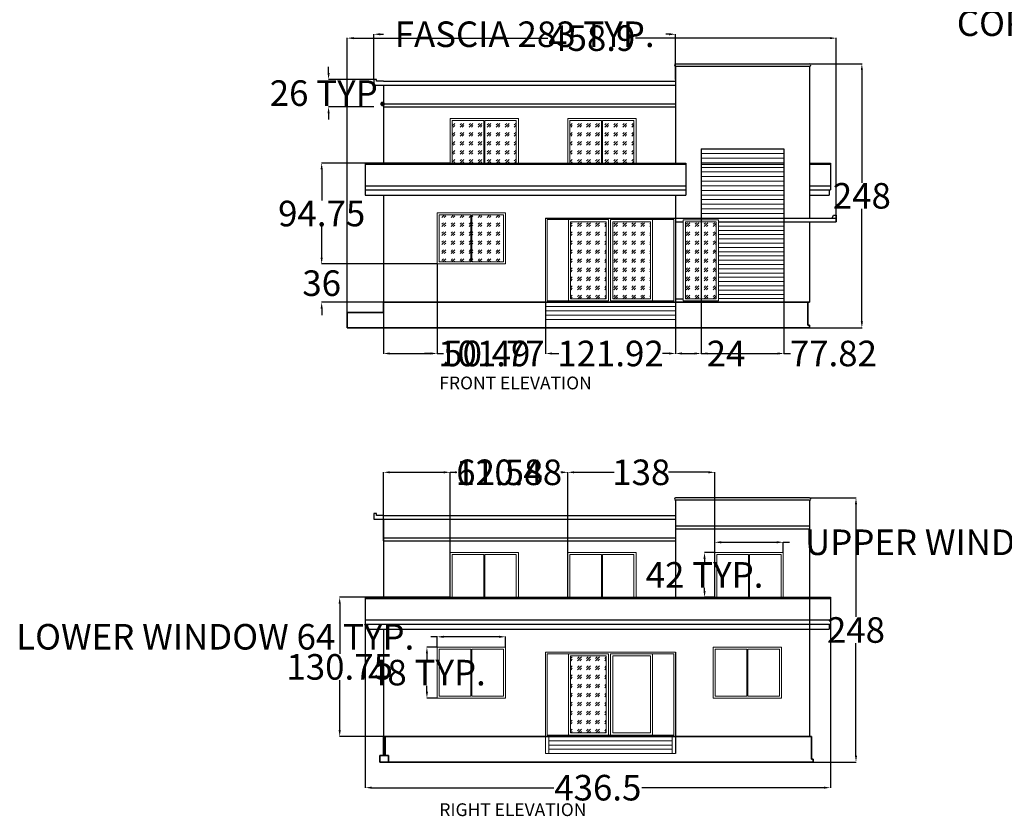
# Model space of a CAD drawing. Units: inches. Extents: x -15 to 1815, y 1023 to 2303.
# Tile 1 of 8: x -15 to 910, y 1024 to 1772. Entities that reach past the tile are written whole.
import ezdxf

# ---------------------------------------------------------------- set-up
doc = ezdxf.new("R2010")
doc.units = ezdxf.units.IN
doc.header["$MEASUREMENT"] = 0
for name, color, linetype, lineweight in [('A-ANNO-DIMS', 2, 'Continuous', 18), ('A-ANNO-TEXT', 7, 'Continuous', 25), ('A-DOOR', 3, 'Continuous', 18), ('A-ELEV', 7, 'Continuous', 25), ('A-ELEV-PATT', 252, 'Continuous', 13), ('A-FLOR-STRS', 3, 'Continuous', 18), ('A-GLAZ', 4, 'Continuous', 18), ('A-GLAZ-PATT', 252, 'Continuous', 13), ('A-ROOF', 7, 'Continuous', 25), ('S-FNDN', 7, 'Continuous', 35)]:
    doc.layers.add(name, color=color, linetype=linetype, lineweight=lineweight)
doc.styles.get("Standard").update_dxf_attribs({"font": 'arial.ttf'})
doc.dimstyles.get("Standard").update_dxf_attribs({"dimtxt": 24, "dimasz": 6, "dimexe": 0.18, "dimexo": 0.0625, "dimgap": 0.09, "dimtad": 0, "dimtih": 1, "dimtoh": 1, "dimdec": 0, "dimzin": 0, "dimdsep": 46, "dimlunit": 3, "dimtxsty": 'Standard', "dimcen": 0.09, "dimadec": 0, "dimazin": 0, "dimtfac": 1, "dimtdec": 0, "dimtofl": 0, "dimtmove": 0, "dimatfit": 3, "dimfxl": 1, "dimtolj": 1, "dimtzin": 0, "dimarcsym": 0})
pattern_1 = [(45, (0, 0), (8.485281, 0), [5, -7]), (45, (2.1213, 0), (8.485281, 0), [2, -10]), (45, (0, 2.1213), (8.485281, 0), [2, -10])]

# ---------------------------------------------------------------- blocks, each defined once
blk = doc.blocks.new('WIN-TWIN-ELEV-42')
for p, q in [((0, 42), (64.17, 42)), ((0, 42), (0, 0)), ((2, 40), (31.58, 40)), ((2, 40), (2, 0)), ((31.58, 0), (31.58, 40)), ((32.58, 40), (62.17, 40)), ((32.58, 0), (32.58, 40)), ((62.17, 40), (62.17, 0)), ((64.17, 42), (64.17, 0))]:
    blk.add_line(p, q)
blk = doc.blocks.new('WIN-TWIN-ELEV-48')
for p, q in [((0, 48), (64.17, 48)), ((0, 48), (0, 0)), ((64.17, 48), (64.17, 0)), ((2, 46), (31.58, 46)), ((2, 46), (2, 2)), ((31.58, 2), (31.58, 46)), ((32.58, 2), (32.58, 46)), ((32.58, 46), (62.17, 46)), ((62.17, 46), (62.17, 2)), ((0, 0), (64.17, 0)), ((2, 2), (31.58, 2)), ((32.58, 2), (62.17, 2))]:
    blk.add_line(p, q)
blk = doc.blocks.new('COPING-ROUND-END')
for p, q in [((1.07, 2.13), (126.89, 2.13)), ((1.07, 0), (126.89, 0))]:
    blk.add_line(p, q)
for centre, start, end in [((1.07, 1.07), 90, 270), ((126.89, 1.07), 270, 90)]:
    blk.add_arc(centre, 1.07, start, end)
blk = doc.blocks.new('FASCIA-PARAPET-ELEV')
for p, q in [((2.47, 25.64), (0, 25.64)), ((0, 25.64), (0, 20.39)), ((0, 20.39), (283.12, 20.39)), ((2.47, 23.92), (2.47, 25.64)), ((8.95, 23.92), (2.47, 23.92)), ((8.95, 23.92), (283.12, 23.92)), ((8.95, 2.89), (283.12, 2.89)), ((8.95, 0), (283.12, 0))]:
    blk.add_line(p, q)
blk = doc.blocks.new('*D41')
at = {"layer": 'A-ANNO-DIMS', "color": 0, "lineweight": -2, "transparency": 16777216}
for p, q in [((637.91, 1272.2), (637.91, 1281.94)), ((643.91, 1281.76), (696.08, 1281.76)), ((702.08, 1272.2), (702.08, 1281.94)), ((702.08, 1281.76), (708.08, 1281.76))]:
    blk.add_line(p, q, dxfattribs=at)
at = {"layer": 'A-ANNO-DIMS', "color": 0, "transparency": 16777216}
for points in [[(643.91, 1282.76), (643.91, 1280.76), (637.91, 1281.76)], [(696.08, 1282.76), (696.08, 1280.76), (702.08, 1281.76)]]:
    blk.add_solid(points, dxfattribs=at)
at = {"layer": 'Defpoints', "color": 0, "transparency": 16777216}
for p in [(702.08, 1281.76), (637.91, 1272.13), (702.08, 1272.13)]:
    blk.add_point(p, dxfattribs=at)
at = {"layer": 'A-ANNO-DIMS', "color": 0, "transparency": 16777216, "insert": (906.58, 1281.76), "char_height": 24, "attachment_point": 5}
blk.add_mtext('\\A1;UPPER WINDOW 64 TYP.', dxfattribs=at)
blk = doc.blocks.new('*D42')
at = {"layer": 'A-ANNO-DIMS', "color": 0, "lineweight": -2, "transparency": 16777216}
for p, q in [((637.85, 1272.13), (628.11, 1272.13)), ((628.29, 1266.13), (628.29, 1263.28)), ((628.29, 1236.13), (628.29, 1238.99)), ((637.85, 1230.13), (628.11, 1230.13))]:
    blk.add_line(p, q, dxfattribs=at)
at = {"layer": 'A-ANNO-DIMS', "color": 0, "transparency": 16777216}
for points in [[(627.29, 1266.13), (629.29, 1266.13), (628.29, 1272.13)], [(627.29, 1236.13), (629.29, 1236.13), (628.29, 1230.13)]]:
    blk.add_solid(points, dxfattribs=at)
at = {"layer": 'Defpoints', "color": 0, "transparency": 16777216}
for p in [(628.29, 1272.13), (637.91, 1272.13), (637.91, 1230.13)]:
    blk.add_point(p, dxfattribs=at)
at = {"layer": 'A-ANNO-DIMS', "color": 0, "transparency": 16777216, "insert": (628.29, 1251.13), "char_height": 24, "attachment_point": 5}
blk.add_mtext('\\A1;42 TYP.', dxfattribs=at)
blk = doc.blocks.new('*D43')
at = {"layer": 'A-ANNO-DIMS', "color": 0, "lineweight": -2, "transparency": 16777216}
for p, q in [((377.32, 1193.01), (371.32, 1193.01)), ((377.32, 1183.44), (377.32, 1193.19)), ((435.49, 1193.01), (383.32, 1193.01)), ((441.49, 1183.44), (441.49, 1193.19))]:
    blk.add_line(p, q, dxfattribs=at)
at = {"layer": 'A-ANNO-DIMS', "color": 0, "transparency": 16777216}
for points in [[(383.32, 1194.01), (383.32, 1192.01), (377.32, 1193.01)], [(435.49, 1194.01), (435.49, 1192.01), (441.49, 1193.01)]]:
    blk.add_solid(points, dxfattribs=at)
at = {"layer": 'Defpoints', "color": 0, "transparency": 16777216}
for p in [(377.32, 1193.01), (377.32, 1183.38), (441.49, 1183.38)]:
    blk.add_point(p, dxfattribs=at)
at = {"layer": 'A-ANNO-DIMS', "color": 0, "transparency": 16777216, "insert": (169.01, 1193.01), "char_height": 24, "attachment_point": 5}
blk.add_mtext('\\A1;LOWER WINDOW 64 TYP.', dxfattribs=at)
blk = doc.blocks.new('*D44')
at = {"layer": 'A-ANNO-DIMS', "color": 0, "lineweight": -2, "transparency": 16777216}
for p, q in [((377.26, 1183.38), (367.52, 1183.38)), ((367.7, 1177.38), (367.7, 1171.73)), ((367.7, 1141.38), (367.7, 1147.04)), ((377.26, 1135.38), (367.52, 1135.38))]:
    blk.add_line(p, q, dxfattribs=at)
at = {"layer": 'A-ANNO-DIMS', "color": 0, "transparency": 16777216}
for points in [[(366.7, 1177.38), (368.7, 1177.38), (367.7, 1183.38)], [(366.7, 1141.38), (368.7, 1141.38), (367.7, 1135.38)]]:
    blk.add_solid(points, dxfattribs=at)
at = {"layer": 'Defpoints', "color": 0, "transparency": 16777216}
for p in [(377.32, 1183.38), (367.7, 1135.38), (377.32, 1135.38)]:
    blk.add_point(p, dxfattribs=at)
at = {"layer": 'A-ANNO-DIMS', "color": 0, "transparency": 16777216, "insert": (367.7, 1159.38), "char_height": 24, "attachment_point": 5}
blk.add_mtext('\\A1;48 TYP.', dxfattribs=at)
blk = doc.blocks.new('*D45')
at = {"layer": 'A-ANNO-DIMS', "color": 0, "lineweight": -2, "transparency": 16777216}
for p, q in [((1138.43, 1769.16), (1132.43, 1769.16)), ((1138.43, 1750.02), (1138.43, 1769.34)), ((1260.44, 1769.16), (1144.43, 1769.16)), ((1266.44, 1750.02), (1266.44, 1769.34))]:
    blk.add_line(p, q, dxfattribs=at)
at = {"layer": 'A-ANNO-DIMS', "color": 0, "transparency": 16777216}
for points in [[(1144.43, 1770.16), (1144.43, 1768.16), (1138.43, 1769.16)], [(1260.44, 1770.16), (1260.44, 1768.16), (1266.44, 1769.16)]]:
    blk.add_solid(points, dxfattribs=at)
at = {"layer": 'Defpoints', "color": 0, "transparency": 16777216}
for p in [(1138.43, 1769.16), (1138.43, 1749.96), (1266.44, 1749.96)]:
    blk.add_point(p, dxfattribs=at)
at = {"layer": 'A-ANNO-DIMS', "color": 0, "transparency": 16777216, "insert": (993.96, 1769.16), "char_height": 24, "attachment_point": 5}
blk.add_mtext('\\A1;COPING 128 TYP.', dxfattribs=at)
blk = doc.blocks.new('*D57')
at = {"layer": 'A-ANNO-DIMS', "color": 0, "lineweight": -2, "transparency": 16777216}
for p, q in [((317.89, 1716.39), (317.89, 1758.98)), ((323.89, 1758.8), (327.1, 1758.8)), ((595.01, 1758.8), (591.8, 1758.8)), ((601.01, 1716.39), (601.01, 1758.98))]:
    blk.add_line(p, q, dxfattribs=at)
at = {"layer": 'A-ANNO-DIMS', "color": 0, "transparency": 16777216}
for points in [[(323.89, 1759.8), (323.89, 1757.8), (317.89, 1758.8)], [(595.01, 1759.8), (595.01, 1757.8), (601.01, 1758.8)]]:
    blk.add_solid(points, dxfattribs=at)
at = {"layer": 'Defpoints', "color": 0, "transparency": 16777216}
for p in [(601.01, 1758.8), (317.89, 1716.33), (601.01, 1716.33)]:
    blk.add_point(p, dxfattribs=at)
at = {"layer": 'A-ANNO-DIMS', "color": 0, "transparency": 16777216, "insert": (459.45, 1758.8), "char_height": 24, "attachment_point": 5}
blk.add_mtext('\\A1;FASCIA 283 TYP.', dxfattribs=at)
blk = doc.blocks.new('*D58')
at = {"layer": 'A-ANNO-DIMS', "color": 0, "lineweight": -2, "transparency": 16777216}
for p, q in [((275.42, 1722.33), (275.42, 1728.33)), ((317.83, 1716.33), (275.24, 1716.33)), ((317.83, 1690.69), (275.24, 1690.69)), ((275.42, 1684.69), (275.42, 1678.69))]:
    blk.add_line(p, q, dxfattribs=at)
at = {"layer": 'A-ANNO-DIMS', "color": 0, "transparency": 16777216}
for points in [[(274.42, 1722.33), (276.42, 1722.33), (275.42, 1716.33)], [(274.42, 1684.69), (276.42, 1684.69), (275.42, 1690.69)]]:
    blk.add_solid(points, dxfattribs=at)
at = {"layer": 'Defpoints', "color": 0, "transparency": 16777216}
for p in [(275.42, 1716.33), (317.89, 1716.33), (317.89, 1690.69)]:
    blk.add_point(p, dxfattribs=at)
at = {"layer": 'A-ANNO-DIMS', "color": 0, "transparency": 16777216, "insert": (275.42, 1703.51), "char_height": 24, "attachment_point": 5}
blk.add_mtext('\\A1;26 TYP.', dxfattribs=at)
blk = doc.blocks.new('*D88')
at = {"layer": 'A-ANNO-DIMS', "color": 0, "lineweight": -2, "transparency": 16777216}
for p, q in [((292.98, 1483.14), (292.98, 1755.33)), ((298.98, 1755.15), (481.34, 1755.15)), ((745.89, 1755.15), (563.53, 1755.15)), ((751.89, 1589.12), (751.89, 1755.33))]:
    blk.add_line(p, q, dxfattribs=at)
at = {"layer": 'A-ANNO-DIMS', "color": 0, "transparency": 16777216}
for points in [[(298.98, 1756.15), (298.98, 1754.15), (292.98, 1755.15)], [(745.89, 1756.15), (745.89, 1754.15), (751.89, 1755.15)]]:
    blk.add_solid(points, dxfattribs=at)
at = {"layer": 'Defpoints', "color": 0, "transparency": 16777216}
for p in [(751.89, 1755.15), (751.89, 1589.05), (292.98, 1483.08)]:
    blk.add_point(p, dxfattribs=at)
at = {"layer": 'A-ANNO-DIMS', "color": 0, "transparency": 16777216, "insert": (522.44, 1755.15), "char_height": 24, "attachment_point": 5}
blk.add_mtext('\\A1;458.9', dxfattribs=at)
blk = doc.blocks.new('*D89')
at = {"layer": 'A-ANNO-DIMS', "color": 0, "lineweight": -2, "transparency": 16777216}
for p, q in [((726.9, 1731.1), (776.12, 1731.1)), ((775.94, 1725.1), (775.94, 1619.43)), ((775.94, 1489.08), (775.94, 1594.75)), ((726.9, 1483.08), (776.12, 1483.08))]:
    blk.add_line(p, q, dxfattribs=at)
at = {"layer": 'A-ANNO-DIMS', "color": 0, "transparency": 16777216}
for points in [[(774.94, 1725.1), (776.94, 1725.1), (775.94, 1731.1)], [(774.94, 1489.08), (776.94, 1489.08), (775.94, 1483.08)]]:
    blk.add_solid(points, dxfattribs=at)
at = {"layer": 'Defpoints', "color": 0, "transparency": 16777216}
for p in [(726.83, 1731.1), (775.94, 1731.1), (726.83, 1483.08)]:
    blk.add_point(p, dxfattribs=at)
at = {"layer": 'A-ANNO-DIMS', "color": 0, "transparency": 16777216, "insert": (775.94, 1607.09), "char_height": 24, "attachment_point": 5}
blk.add_mtext('\\A1;248', dxfattribs=at)
blk = doc.blocks.new('*D90')
at = {"layer": 'A-ANNO-DIMS', "color": 0, "lineweight": -2, "transparency": 16777216}
for p, q in [((377.32, 1543.01), (377.32, 1458.85)), ((326.83, 1507.01), (326.83, 1458.85)), ((332.83, 1459.03), (371.32, 1459.03)), ((377.32, 1459.03), (383.32, 1459.03))]:
    blk.add_line(p, q, dxfattribs=at)
at = {"layer": 'A-ANNO-DIMS', "color": 0, "transparency": 16777216}
for points in [[(332.83, 1460.03), (332.83, 1458.03), (326.83, 1459.03)], [(371.32, 1460.03), (371.32, 1458.03), (377.32, 1459.03)]]:
    blk.add_solid(points, dxfattribs=at)
at = {"layer": 'Defpoints', "color": 0, "transparency": 16777216}
for p in [(377.32, 1543.08), (326.83, 1507.08), (377.32, 1459.03)]:
    blk.add_point(p, dxfattribs=at)
at = {"layer": 'A-ANNO-DIMS', "color": 0, "transparency": 16777216, "insert": (423.93, 1459.03), "char_height": 24, "attachment_point": 5}
blk.add_mtext('\\A1;50.49', dxfattribs=at)
blk = doc.blocks.new('*D91')
at = {"layer": 'A-ANNO-DIMS', "color": 0, "lineweight": -2, "transparency": 16777216}
for p, q in [((377.320354, 1543.014849), (377.320354, 1458.847349)), ((479.094066, 1507.014849), (479.094066, 1458.847349)), ((371.320354, 1459.027349), (365.320354, 1459.027349)), ((485.094066, 1459.027349), (491.094066, 1459.027349))]:
    blk.add_line(p, q, dxfattribs=at)
at = {"layer": 'A-ANNO-DIMS', "color": 0, "transparency": 16777216}
for points in [[(371.320354, 1460.027349), (371.320354, 1458.027349), (377.320354, 1459.027349)], [(485.094066, 1460.027349), (485.094066, 1458.027349), (479.094066, 1459.027349)]]:
    blk.add_solid(points, dxfattribs=at)
at = {"layer": 'Defpoints', "color": 0, "transparency": 16777216}
for p in [(377.320354, 1543.077349), (479.094066, 1507.077349), (479.094066, 1459.027349)]:
    blk.add_point(p, dxfattribs=at)
at = {"layer": 'A-ANNO-DIMS', "color": 0, "transparency": 16777216, "insert": (428.20721, 1459.027349), "char_height": 24, "attachment_point": 5}
blk.add_mtext('\\A1;101.77', dxfattribs=at)
blk = doc.blocks.new('*D92')
at = {"layer": 'A-ANNO-DIMS', "color": 0, "lineweight": -2, "transparency": 16777216}
for p, q in [((479.09, 1507.01), (479.09, 1458.85)), ((601.01, 1507.01), (601.01, 1458.85)), ((485.09, 1459.03), (491.4, 1459.03)), ((595.01, 1459.03), (588.71, 1459.03))]:
    blk.add_line(p, q, dxfattribs=at)
at = {"layer": 'A-ANNO-DIMS', "color": 0, "transparency": 16777216}
for points in [[(485.09, 1460.03), (485.09, 1458.03), (479.09, 1459.03)], [(595.01, 1460.03), (595.01, 1458.03), (601.01, 1459.03)]]:
    blk.add_solid(points, dxfattribs=at)
at = {"layer": 'Defpoints', "color": 0, "transparency": 16777216}
for p in [(479.09, 1507.08), (601.01, 1507.08), (601.01, 1459.03)]:
    blk.add_point(p, dxfattribs=at)
at = {"layer": 'A-ANNO-DIMS', "color": 0, "transparency": 16777216, "insert": (540.05, 1459.03), "char_height": 24, "attachment_point": 5}
blk.add_mtext('\\A1;121.92', dxfattribs=at)
blk = doc.blocks.new('*D93')
at = {"layer": 'A-ANNO-DIMS', "color": 0, "lineweight": -2, "transparency": 16777216}
for p, q in [((625.01, 1651.01), (625.01, 1458.85)), ((601.01, 1507.01), (601.01, 1458.85)), ((607.01, 1459.03), (619.01, 1459.03)), ((625.01, 1459.03), (631.01, 1459.03))]:
    blk.add_line(p, q, dxfattribs=at)
at = {"layer": 'A-ANNO-DIMS', "color": 0, "transparency": 16777216}
for points in [[(607.01, 1460.03), (607.01, 1458.03), (601.01, 1459.03)], [(619.01, 1460.03), (619.01, 1458.03), (625.01, 1459.03)]]:
    blk.add_solid(points, dxfattribs=at)
at = {"layer": 'Defpoints', "color": 0, "transparency": 16777216}
for p in [(625.01, 1651.08), (601.01, 1507.08), (625.01, 1459.03)]:
    blk.add_point(p, dxfattribs=at)
at = {"layer": 'A-ANNO-DIMS', "color": 0, "transparency": 16777216, "insert": (648.45, 1459.03), "char_height": 24, "attachment_point": 5}
blk.add_mtext('\\A1;24', dxfattribs=at)
blk = doc.blocks.new('*D94')
at = {"layer": 'A-ANNO-DIMS', "color": 0, "lineweight": -2, "transparency": 16777216}
for p, q in [((625.01, 1651.01), (625.01, 1458.85)), ((702.83, 1507.01), (702.83, 1458.85)), ((631.01, 1459.03), (696.83, 1459.03)), ((702.83, 1459.03), (708.83, 1459.03))]:
    blk.add_line(p, q, dxfattribs=at)
at = {"layer": 'A-ANNO-DIMS', "color": 0, "transparency": 16777216}
for points in [[(631.01, 1460.03), (631.01, 1458.03), (625.01, 1459.03)], [(696.83, 1460.03), (696.83, 1458.03), (702.83, 1459.03)]]:
    blk.add_solid(points, dxfattribs=at)
at = {"layer": 'Defpoints', "color": 0, "transparency": 16777216}
for p in [(625.01, 1651.08), (702.83, 1507.08), (702.83, 1459.03)]:
    blk.add_point(p, dxfattribs=at)
at = {"layer": 'A-ANNO-DIMS', "color": 0, "transparency": 16777216, "insert": (749.2, 1459.03), "char_height": 24, "attachment_point": 5}
blk.add_mtext('\\A1;77.82', dxfattribs=at)
blk = doc.blocks.new('*D95')
at = {"layer": 'A-ANNO-DIMS', "color": 0, "lineweight": -2, "transparency": 16777216}
for p, q in [((268.932113, 1549.077349), (268.932113, 1555.077349)), ((377.257854, 1543.077349), (268.752113, 1543.077349)), ((326.772175, 1507.077349), (268.752113, 1507.077349)), ((268.932113, 1501.077349), (268.932113, 1495.077349))]:
    blk.add_line(p, q, dxfattribs=at)
at = {"layer": 'A-ANNO-DIMS', "color": 0, "transparency": 16777216}
for points in [[(267.932113, 1549.077349), (269.932113, 1549.077349), (268.932113, 1543.077349)], [(267.932113, 1501.077349), (269.932113, 1501.077349), (268.932113, 1507.077349)]]:
    blk.add_solid(points, dxfattribs=at)
at = {"layer": 'Defpoints', "color": 0, "transparency": 16777216}
for p in [(268.932113, 1543.077349), (377.320354, 1543.077349), (326.834675, 1507.077349)]:
    blk.add_point(p, dxfattribs=at)
at = {"layer": 'A-ANNO-DIMS', "color": 0, "transparency": 16777216, "insert": (268.932113, 1525.077349), "char_height": 24, "attachment_point": 5}
blk.add_mtext('\\A1;36', dxfattribs=at)
blk = doc.blocks.new('*D96')
at = {"layer": 'A-ANNO-DIMS', "color": 0, "lineweight": -2, "transparency": 16777216}
for p, q in [((389.35, 1637.83), (268.75, 1637.83)), ((268.93, 1631.83), (268.93, 1602.8)), ((268.93, 1549.08), (268.93, 1578.11)), ((377.26, 1543.08), (268.75, 1543.08))]:
    blk.add_line(p, q, dxfattribs=at)
at = {"layer": 'A-ANNO-DIMS', "color": 0, "transparency": 16777216}
for points in [[(267.93, 1631.83), (269.93, 1631.83), (268.93, 1637.83)], [(267.93, 1549.08), (269.93, 1549.08), (268.93, 1543.08)]]:
    blk.add_solid(points, dxfattribs=at)
at = {"layer": 'Defpoints', "color": 0, "transparency": 16777216}
for p in [(268.93, 1637.83), (389.41, 1637.83), (377.32, 1543.08)]:
    blk.add_point(p, dxfattribs=at)
at = {"layer": 'A-ANNO-DIMS', "color": 0, "transparency": 16777216, "insert": (268.93, 1590.45), "char_height": 24, "attachment_point": 5}
blk.add_mtext('\\A1;94.75', dxfattribs=at)
blk = doc.blocks.new('*D97')
at = {"layer": 'A-ANNO-DIMS', "color": 0, "lineweight": -2, "transparency": 16777216}
for p, q in [((309.87, 1230.07), (309.87, 1051.15)), ((746.38, 1230.07), (746.38, 1051.15)), ((315.87, 1051.33), (486.97, 1051.33)), ((740.38, 1051.33), (569.28, 1051.33))]:
    blk.add_line(p, q, dxfattribs=at)
at = {"layer": 'A-ANNO-DIMS', "color": 0, "transparency": 16777216}
for points in [[(315.87, 1052.33), (315.87, 1050.33), (309.87, 1051.33)], [(740.38, 1052.33), (740.38, 1050.33), (746.38, 1051.33)]]:
    blk.add_solid(points, dxfattribs=at)
at = {"layer": 'Defpoints', "color": 0, "transparency": 16777216}
for p in [(309.87, 1230.13), (746.38, 1230.13), (746.38, 1051.33)]:
    blk.add_point(p, dxfattribs=at)
at = {"layer": 'A-ANNO-DIMS', "color": 0, "transparency": 16777216, "insert": (528.13, 1051.33), "char_height": 24, "attachment_point": 5}
blk.add_mtext('\\A1;436.5', dxfattribs=at)
blk = doc.blocks.new('*D98')
at = {"layer": 'A-ANNO-DIMS', "color": 0, "lineweight": -2, "transparency": 16777216}
for p, q in [((726.9, 1323.41), (770.61, 1323.41)), ((770.43, 1317.41), (770.43, 1211.74)), ((770.43, 1081.38), (770.43, 1187.05)), ((730.36, 1075.38), (770.61, 1075.38))]:
    blk.add_line(p, q, dxfattribs=at)
at = {"layer": 'A-ANNO-DIMS', "color": 0, "transparency": 16777216}
for points in [[(769.43, 1317.41), (771.43, 1317.41), (770.43, 1323.41)], [(769.43, 1081.38), (771.43, 1081.38), (770.43, 1075.38)]]:
    blk.add_solid(points, dxfattribs=at)
at = {"layer": 'Defpoints', "color": 0, "transparency": 16777216}
for p in [(726.83, 1323.41), (770.43, 1323.41), (730.3, 1075.38)]:
    blk.add_point(p, dxfattribs=at)
at = {"layer": 'A-ANNO-DIMS', "color": 0, "transparency": 16777216, "insert": (770.43, 1199.39), "char_height": 24, "attachment_point": 5}
blk.add_mtext('\\A1;248', dxfattribs=at)
blk = doc.blocks.new('*D99')
at = {"layer": 'A-ANNO-DIMS', "color": 0, "lineweight": -2, "transparency": 16777216}
for p, q in [((326.83, 1283.06), (326.83, 1347.64)), ((332.83, 1347.46), (383.41, 1347.46)), ((389.41, 1230.2), (389.41, 1347.64)), ((389.41, 1347.46), (395.41, 1347.46))]:
    blk.add_line(p, q, dxfattribs=at)
at = {"layer": 'A-ANNO-DIMS', "color": 0, "transparency": 16777216}
for points in [[(332.83, 1348.46), (332.83, 1346.46), (326.83, 1347.46)], [(383.41, 1348.46), (383.41, 1346.46), (389.41, 1347.46)]]:
    blk.add_solid(points, dxfattribs=at)
at = {"layer": 'Defpoints', "color": 0, "transparency": 16777216}
for p in [(389.41, 1347.46), (326.83, 1282.99), (389.41, 1230.13)]:
    blk.add_point(p, dxfattribs=at)
at = {"layer": 'A-ANNO-DIMS', "color": 0, "transparency": 16777216, "insert": (436.09, 1347.46), "char_height": 24, "attachment_point": 5}
blk.add_mtext('\\A1;62.58', dxfattribs=at)
blk = doc.blocks.new('*D100')
at = {"layer": 'A-ANNO-DIMS', "color": 0, "lineweight": -2, "transparency": 16777216}
for p, q in [((389.41, 1230.2), (389.41, 1347.64)), ((395.41, 1347.46), (395.85, 1347.46)), ((493.9, 1347.46), (493.46, 1347.46)), ((499.9, 1230.2), (499.9, 1347.64))]:
    blk.add_line(p, q, dxfattribs=at)
at = {"layer": 'A-ANNO-DIMS', "color": 0, "transparency": 16777216}
for points in [[(395.41, 1348.46), (395.41, 1346.46), (389.41, 1347.46)], [(493.9, 1348.46), (493.9, 1346.46), (499.9, 1347.46)]]:
    blk.add_solid(points, dxfattribs=at)
at = {"layer": 'Defpoints', "color": 0, "transparency": 16777216}
for p in [(499.9, 1347.46), (389.41, 1230.13), (499.9, 1230.13)]:
    blk.add_point(p, dxfattribs=at)
at = {"layer": 'A-ANNO-DIMS', "color": 0, "transparency": 16777216, "insert": (444.66, 1347.46), "char_height": 24, "attachment_point": 5}
blk.add_mtext('\\A1;110.48', dxfattribs=at)
blk = doc.blocks.new('*D101')
at = {"layer": 'A-ANNO-DIMS', "color": 0, "lineweight": -2, "transparency": 16777216}
for p, q in [((499.9, 1230.2), (499.9, 1347.64)), ((505.9, 1347.46), (543.41, 1347.46)), ((631.91, 1347.46), (594.4, 1347.46)), ((637.91, 1230.2), (637.91, 1347.64))]:
    blk.add_line(p, q, dxfattribs=at)
at = {"layer": 'A-ANNO-DIMS', "color": 0, "transparency": 16777216}
for points in [[(505.9, 1348.46), (505.9, 1346.46), (499.9, 1347.46)], [(631.91, 1348.46), (631.91, 1346.46), (637.91, 1347.46)]]:
    blk.add_solid(points, dxfattribs=at)
at = {"layer": 'Defpoints', "color": 0, "transparency": 16777216}
for p in [(637.91, 1347.46), (499.9, 1230.13), (637.91, 1230.13)]:
    blk.add_point(p, dxfattribs=at)
at = {"layer": 'A-ANNO-DIMS', "color": 0, "transparency": 16777216, "insert": (568.9, 1347.46), "char_height": 24, "attachment_point": 5}
blk.add_mtext('\\A1;138', dxfattribs=at)
blk = doc.blocks.new('*D102')
at = {"layer": 'A-ANNO-DIMS', "color": 0, "lineweight": -2, "transparency": 16777216}
for p, q in [((389.35, 1230.13), (285.64, 1230.13)), ((285.82, 1224.13), (285.82, 1177.11)), ((285.82, 1105.38), (285.82, 1152.41)), ((326.77, 1099.38), (285.64, 1099.38))]:
    blk.add_line(p, q, dxfattribs=at)
at = {"layer": 'A-ANNO-DIMS', "color": 0, "transparency": 16777216}
for points in [[(284.82, 1224.13), (286.82, 1224.13), (285.82, 1230.13)], [(284.82, 1105.38), (286.82, 1105.38), (285.82, 1099.38)]]:
    blk.add_solid(points, dxfattribs=at)
at = {"layer": 'Defpoints', "color": 0, "transparency": 16777216}
for p in [(285.82, 1230.13), (389.41, 1230.13), (326.83, 1099.38)]:
    blk.add_point(p, dxfattribs=at)
at = {"layer": 'A-ANNO-DIMS', "color": 0, "transparency": 16777216, "insert": (285.82, 1164.76), "char_height": 24, "attachment_point": 5}
blk.add_mtext('\\A1;130.75', dxfattribs=at)

msp = doc.modelspace()

# ---------------------------------------------------------------- hatches: boundary and pattern name
at = {"layer": 'A-ELEV-PATT'}
h = msp.add_hatch(dxfattribs=at)
h.set_pattern_fill('ANSI31', color=256, scale=34.6701, angle=-45, style=0)
h.paths.add_polyline_path([(625.0103, 1586.2036), (702.8347, 1586.2036), (702.8347, 1651.0773), (625.0103, 1651.0773)])
h = msp.add_hatch(dxfattribs=at)
h.set_pattern_fill('ANSI31', color=256, scale=32.0538, angle=-45, style=0)
h.paths.add_polyline_path([(641.2936, 1507.0773), (702.8347, 1507.0773), (702.8347, 1582.655), (641.2936, 1582.655)])
at = {"layer": 'A-GLAZ-PATT'}
h = msp.add_hatch(dxfattribs=at)
h.set_pattern_fill('GOST_GLASS', color=256)
h.set_pattern_definition(pattern_1)
h.paths.add_polyline_path([(639.2936, 1582.655), (610.3359, 1582.655), (610.3359, 1510.5025), (639.2936, 1510.5025)])
h.paths.add_polyline_path([(439.4857, 1589.0773), (409.903, 1589.0773), (409.903, 1545.0773), (439.4857, 1545.0773)])
h.paths.add_polyline_path([(408.903, 1589.0773), (379.3204, 1589.0773), (379.3204, 1545.0773), (408.903, 1545.0773)])
h.paths.add_polyline_path([(451.5798, 1677.8282), (421.9972, 1677.8282), (421.9972, 1637.8282), (451.5798, 1637.8282)])
h.paths.add_polyline_path([(420.9972, 1677.8282), (391.4145, 1677.8282), (391.4145, 1637.8282), (420.9972, 1637.8282)])
h.paths.add_polyline_path([(531.4796, 1677.8282), (501.897, 1677.8282), (501.897, 1637.8282), (531.4796, 1637.8282)])
h.paths.add_polyline_path([(562.0623, 1677.8282), (532.4796, 1677.8282), (532.4796, 1637.8282), (562.0623, 1637.8282)])
h.paths.add_polyline_path([(577.5602, 1582.7959), (542.0522, 1582.7959), (542.0522, 1510.485), (577.5602, 1510.485)])
h = msp.add_hatch(dxfattribs=at)
h.set_pattern_fill('GOST_GLASS', color=256)
h.set_pattern_definition(pattern_1)
h.paths.add_polyline_path([(536.0522, 1582.7959), (502.5441, 1582.7959), (502.5441, 1510.485), (536.0522, 1510.485)])
h = msp.add_hatch(dxfattribs=at)
h.set_pattern_fill('GOST_GLASS', color=256)
h.set_pattern_definition([(45, (-1e-13, -407.6953), (8.485281, 0), [5, -7]), (45, (2.1213, -407.6953), (8.485281, 0), [2, -10]), (45, (-1e-13, -405.574), (8.485281, 0), [2, -10])])
h.paths.add_polyline_path([(536.0522, 1175.1006), (502.5441, 1175.1006), (502.5441, 1102.7897), (536.0522, 1102.7897)])

# ---------------------------------------------------------------- linework, layer by layer
at = {"layer": 'A-DOOR'}
for p, q in [((500.5441, 1584.7959), (500.5441, 1508.485)), ((502.5441, 1582.7959), (502.5441, 1510.485)), ((536.0522, 1510.485), (536.0522, 1582.7959)), ((538.0522, 1508.485), (538.0522, 1584.7959)), ((540.0522, 1508.485), (540.0522, 1584.7959)), ((542.0522, 1510.485), (542.0522, 1582.7959)), ((577.5602, 1582.7959), (577.5602, 1510.485)), ((579.5602, 1584.7959), (579.5602, 1508.485)), ((479.0941, 1178.5083), (601.0103, 1178.5083)), ((500.5441, 1177.1006), (500.5441, 1100.7897)), ((502.5441, 1175.1006), (502.5441, 1102.7897)), ((536.0522, 1102.7897), (536.0522, 1175.1006)), ((538.0522, 1100.7897), (538.0522, 1177.1006)), ((540.0522, 1100.7897), (540.0522, 1177.1006)), ((542.0522, 1102.7897), (542.0522, 1175.1006)), ((577.5602, 1175.1006), (577.5602, 1102.7897)), ((579.5602, 1177.1006), (579.5602, 1100.7897))]:
    msp.add_line(p, q, dxfattribs=at)
msp.add_lwpolyline([(479.0941, 1507.0773), (601.0103, 1507.0773), (601.0103, 1586.2036), (479.0941, 1586.2036)], close=True, dxfattribs=at)
for points in [[(538.0522, 1584.7959), (480.5017, 1584.7959), (480.5017, 1508.485), (538.0522, 1508.485)], [(536.0522, 1582.7959), (502.5441, 1582.7959)], [(579.5602, 1584.7959), (540.0522, 1584.7959)], [(540.0522, 1508.485), (599.6026, 1508.485), (599.6026, 1584.7959), (542.0522, 1584.7959)], [(577.5602, 1582.7959), (542.0522, 1582.7959)], [(502.5441, 1510.485), (536.0522, 1510.485)], [(540.0522, 1508.485), (579.5602, 1508.485)], [(542.0522, 1510.485), (577.5602, 1510.485)], [(601.0103, 1178.5083), (601.0103, 1178.5083), (479.0941, 1178.5083), (479.0941, 1099.382), (601.0103, 1099.382), (601.0103, 1174.9596)], [(538.0522, 1177.1006), (480.5017, 1177.1006), (480.5017, 1100.7897), (540.0522, 1100.7897)], [(536.0522, 1175.1006), (502.5441, 1175.1006)], [(540.0522, 1100.7897), (599.6026, 1100.7897), (599.6026, 1177.1006), (542.0522, 1177.1006)], [(579.5602, 1177.1006), (540.0522, 1177.1006)], [(577.5602, 1175.1006), (542.0522, 1175.1006)], [(502.5441, 1102.7897), (536.0522, 1102.7897)], [(540.0522, 1100.7897), (579.5602, 1100.7897)], [(542.0522, 1102.7897), (577.5602, 1102.7897)]]:
    msp.add_lwpolyline(points, dxfattribs=at)
at = {"layer": 'A-ELEV'}
for p, q in [((601.0103, 1728.9687), (601.0103, 1636.7189)), ((726.8347, 1728.9687), (726.8347, 1586.2036)), ((326.8347, 1711.0773), (326.8347, 1637.8282)), ((625.0103, 1651.0773), (702.8347, 1651.0773)), ((625.0103, 1651.0773), (625.0103, 1586.2036)), ((702.8347, 1651.0773), (702.8347, 1507.0773)), ((309.873, 1637.8282), (610.7121, 1637.8282)), ((309.873, 1637.8282), (309.873, 1607.8282)), ((309.873, 1637.8282), (610.7121, 1637.8282)), ((309.873, 1636.7189), (610.7121, 1636.7189)), ((610.7121, 1637.8282), (610.7121, 1607.8282)), ((625.0103, 1636.7189), (702.8347, 1636.7189)), ((726.8347, 1637.8282), (746.3784, 1637.8282)), ((726.8347, 1637.8282), (746.3784, 1637.8282)), ((726.8347, 1636.7189), (746.3784, 1636.7189)), ((746.3784, 1637.8282), (746.3784, 1612.6439)), ((309.873, 1616.5914), (610.7121, 1616.5914)), ((309.873, 1612.6439), (610.7121, 1612.6439)), ((726.8347, 1616.5914), (746.3784, 1616.5914)), ((726.8347, 1612.6439), (746.3784, 1612.6439)), ((745.2075, 1612.6439), (745.2075, 1607.8282)), ((309.873, 1607.8282), (610.7121, 1607.8282)), ((326.8347, 1607.8282), (326.8347, 1497.6672)), ((601.0103, 1607.8282), (601.0103, 1491.0773)), ((726.8347, 1607.8282), (745.2075, 1607.8282)), ((479.0941, 1586.2036), (751.6243, 1586.2036)), ((601.0103, 1582.655), (608.3359, 1582.655)), ((641.2936, 1582.655), (751.8892, 1582.655)), ((726.8347, 1582.655), (726.8347, 1507.0773)), ((748.121, 1586.2036), (749.3011, 1589.0526)), ((749.3011, 1589.0526), (751.8892, 1589.0526)), ((751.6243, 1589.0526), (751.6243, 1582.655)), ((751.8892, 1589.0526), (751.8892, 1582.655)), ((601.0103, 1510.5025), (608.3359, 1510.5025)), ((601.0103, 1321.2734), (601.0103, 1230.1328)), ((726.8347, 1321.2734), (726.8347, 1178.5083)), ((326.8347, 1303.382), (326.8347, 1230.1328)), ((309.873, 1230.1328), (610.7121, 1230.1328)), ((309.873, 1230.1328), (309.873, 1204.9486)), ((309.873, 1230.1328), (726.8347, 1230.1328)), ((726.8347, 1230.1328), (746.3784, 1230.1328)), ((726.8347, 1230.1328), (746.3784, 1230.1328)), ((746.3784, 1230.1328), (746.3784, 1204.9486)), ((309.873, 1229.0236), (726.8347, 1229.0236)), ((726.8347, 1229.0236), (746.3784, 1229.0236)), ((309.873, 1208.896), (726.8347, 1208.896)), ((309.873, 1204.9486), (726.8347, 1204.9486)), ((312.3523, 1200.1328), (312.3523, 1204.9486)), ((726.8347, 1208.896), (746.3784, 1208.896)), ((726.8347, 1204.9486), (746.3784, 1204.9486)), ((745.2075, 1204.9486), (745.2075, 1200.1328)), ((312.3523, 1200.1328), (726.8347, 1200.1328)), ((326.8347, 1200.1328), (326.8347, 1081.6107)), ((726.8347, 1200.1328), (745.2075, 1200.1328)), ((726.8347, 1200.1328), (726.8347, 1099.382)), ((601.0103, 1178.5083), (601.0103, 1083.382))]:
    msp.add_line(p, q, dxfattribs=at)
at = {"layer": 'A-FLOR-STRS'}
for p, q in [((479.0941, 1507.0773), (479.0941, 1491.0773)), ((479.0941, 1503.0076), (601.0103, 1503.0076)), ((479.0941, 1499.0773), (601.0103, 1499.0773)), ((479.0941, 1495.0773), (601.0103, 1495.0773)), ((479.0941, 1491.0773), (601.0103, 1491.0773)), ((479.0941, 1099.382), (479.0941, 1083.382)), ((482.0505, 1099.382), (482.0505, 1083.382)), ((482.0505, 1095.3122), (598.0539, 1095.3122)), ((482.0505, 1091.382), (598.0539, 1091.382)), ((598.0539, 1099.382), (598.0539, 1083.382)), ((479.0941, 1083.382), (601.0103, 1083.382)), ((482.0505, 1087.382), (598.0539, 1087.382))]:
    msp.add_line(p, q, dxfattribs=at)
at = {"layer": 'A-GLAZ'}
for p, q in [((610.3359, 1582.655), (639.2936, 1582.655)), ((610.3359, 1510.5025), (639.2936, 1510.5025))]:
    msp.add_line(p, q, dxfattribs=at)
for points in [[(608.3359, 1508.5025), (641.2936, 1508.5025), (641.2936, 1584.655), (608.3359, 1584.655)], [(610.3359, 1510.5025), (639.2936, 1510.5025), (639.2936, 1582.655), (610.3359, 1582.655)]]:
    msp.add_lwpolyline(points, close=True, dxfattribs=at)
at = {"layer": 'A-ROOF'}
for p, q in [((601.0103, 1297.2072), (726.8347, 1297.2072)), ((601.0103, 1294.3147), (726.8347, 1294.3147))]:
    msp.add_line(p, q, dxfattribs=at)
at = {"layer": 'S-FNDN'}
for p, q in [((326.8347, 1507.0773), (601.0103, 1507.0773)), ((326.8347, 1497.6672), (326.8347, 1507.0773)), ((601.0103, 1507.0773), (726.8347, 1507.0773)), ((725.2983, 1485.6878), (725.2983, 1507.0773)), ((292.9821, 1483.0773), (292.9821, 1497.6672)), ((292.9821, 1497.6672), (326.8347, 1497.6672)), ((326.8347, 1483.0773), (292.9821, 1483.0773)), ((326.8347, 1483.0773), (726.8347, 1483.0773)), ((326.8347, 1483.0773), (601.0103, 1483.0773)), ((720.3821, 1483.0773), (726.8347, 1483.0773)), ((726.8347, 1485.6878), (725.2983, 1485.6878)), ((726.8347, 1483.0773), (726.8347, 1485.6878)), ((726.8347, 1483.0773), (726.8347, 1485.6878)), ((326.8347, 1099.382), (601.0103, 1099.382)), ((326.8347, 1081.6107), (326.8347, 1099.382)), ((328.418, 1081.6107), (328.418, 1099.382)), ((601.0103, 1099.382), (728.7646, 1099.382)), ((728.7646, 1077.9925), (728.7646, 1099.382)), ((323.3874, 1075.382), (323.3874, 1081.6107)), ((323.3874, 1081.6107), (328.418, 1081.6107)), ((331.7004, 1081.6107), (326.6698, 1081.6107)), ((331.7004, 1075.382), (331.7004, 1081.6107)), ((326.8347, 1075.382), (323.3874, 1075.382)), ((326.8347, 1075.382), (730.301, 1075.382)), ((326.8347, 1075.382), (601.0103, 1075.382)), ((720.3821, 1075.382), (730.301, 1075.382)), ((730.301, 1077.9925), (728.7646, 1077.9925)), ((730.301, 1075.382), (730.301, 1077.9925))]:
    msp.add_line(p, q, dxfattribs=at)

# ---------------------------------------------------------------- block references
at = {"layer": 'A-GLAZ'}
for name, p in [('WIN-TWIN-ELEV-42', (389.4145, 1637.8282)), ('WIN-TWIN-ELEV-42', (499.897, 1637.8282)), ('WIN-TWIN-ELEV-48', (377.3204, 1543.0773)), ('WIN-TWIN-ELEV-42', (389.4145, 1230.1328)), ('WIN-TWIN-ELEV-42', (499.897, 1230.1328)), ('WIN-TWIN-ELEV-42', (637.9105, 1230.1328))]:
    msp.add_blockref(name, p, dxfattribs=at)
at = {"layer": 'A-GLAZ', "rotation": 180}
for p in [(441.4857, 1183.382), (700.5595, 1183.382)]:
    msp.add_blockref('WIN-TWIN-ELEV-48', p, dxfattribs=at)
at = {"layer": 'A-ROOF'}
for name, p in [('COPING-ROUND-END', (599.9444, 1728.9687)), ('FASCIA-PARAPET-ELEV', (317.8894, 1690.688)), ('FASCIA-PARAPET-ELEV', (317.8894, 1282.9927))]:
    msp.add_blockref(name, p, dxfattribs=at)
at = {"layer": 'A-ROOF', "rotation": 180}
msp.add_blockref('COPING-ROUND-END', (727.9006, 1323.4052), dxfattribs=at)

# ---------------------------------------------------------------- texts
at = {"layer": 'A-ANNO-TEXT'}
for s, p in [('FRONT ELEVATION', (379.3855, 1425.3698)), ('RIGHT ELEVATION', (379.3855, 1024.6485))]:
    msp.add_text(s, height=12, dxfattribs=at).set_placement(p)

# ---------------------------------------------------------------- dimensions: what is measured, and where the dimension line sits
at = {"layer": 'A-ANNO-DIMS'}
for base, p1, p2, angle, text, picture, middle in [((1138.4338, 1769.1591), (1266.4376, 1749.9585), (1138.4338, 1749.9585), 180, 'COPING <> TYP.', '*D45', (993.9591, 1769.1591)), ((275.4212, 1716.3286), (317.8894, 1690.688), (317.8894, 1716.3286), 90, '<> TYP.', '*D58', (275.4212, 1703.5083)), ((628.2857, 1272.1328), (637.9105, 1230.1328), (637.9105, 1272.1328), 90, '<> TYP.', '*D42', (628.2857, 1251.1328)), ((377.3204, 1193.0068), (441.4857, 1183.382), (377.3204, 1183.382), 180, 'LOWER WINDOW <> TYP.', '*D43', (169.0066, 1193.0068)), ((367.6956, 1135.382), (377.3204, 1183.382), (377.3204, 1135.382), 270, '<> TYP.', '*D44', (367.6956, 1159.382))]:
    dim = msp.add_linear_dim(base=base, p1=p1, p2=p2, angle=angle, text=text, dimstyle='Standard', override={"dimdec": 0, "dimlfac": 1, "dimrnd": 0, "dimzin": 0, "dimdsep": 46, "dimlunit": 2}, dxfattribs=at)
    dim.commit()
    dim.dimension.update_dxf_attribs({"geometry": picture, "text_midpoint": middle})
for base, p1, p2, text, picture, middle in [((601.0103, 1758.7967), (317.8894, 1716.3286), (601.0103, 1716.3286), 'FASCIA <> TYP.', '*D57', (459.4498, 1758.7967)), ((702.0758, 1281.7576), (637.9105, 1272.1328), (702.0758, 1272.1328), 'UPPER WINDOW <> TYP.', '*D41', (906.5833, 1281.7576))]:
    dim = msp.add_linear_dim(base=base, p1=p1, p2=p2, text=text, dimstyle='Standard', override={"dimdec": 0, "dimlfac": 1, "dimrnd": 0, "dimzin": 0, "dimdsep": 46, "dimlunit": 2}, dxfattribs=at)
    dim.commit()
    dim.dimension.update_dxf_attribs({"geometry": picture, "text_midpoint": middle})
for base, p1, p2, override, picture, middle in [((751.8892, 1755.1505), (292.9821, 1483.0773), (751.8892, 1589.0526), {"dimdec": 1, "dimlfac": 1, "dimrnd": 0, "dimzin": 0, "dimdsep": 46, "dimlunit": 2}, '*D88', (522.4357, 1755.1505)), ((625.0103, 1459.0273), (601.0103, 1507.0773), (625.0103, 1651.0773), {"dimdec": 0, "dimlfac": 1, "dimrnd": 0, "dimzin": 0, "dimdsep": 46, "dimlunit": 2}, '*D93', (648.4454, 1459.0273)), ((702.8347, 1459.0273), (625.0103, 1651.0773), (702.8347, 1507.0773), {"dimdec": 2, "dimlfac": 1, "dimrnd": 0, "dimzin": 0, "dimdsep": 46, "dimlunit": 2}, '*D94', (749.1975, 1459.0273)), ((377.3204, 1459.0273), (326.8347, 1507.0773), (377.3204, 1543.0773), {"dimdec": 2, "dimlfac": 1, "dimrnd": 0, "dimzin": 0, "dimdsep": 46, "dimlunit": 2}, '*D90', (423.9288, 1459.0273)), ((479.0941, 1459.0273), (377.3204, 1543.0773), (479.0941, 1507.0773), {"dimdec": 2, "dimlfac": 1, "dimrnd": 0, "dimzin": 0, "dimdsep": 46, "dimlunit": 2}, '*D91', (428.2072, 1459.0273)), ((601.0103, 1459.0273), (479.0941, 1507.0773), (601.0103, 1507.0773), {"dimdec": 2, "dimlfac": 1, "dimrnd": 0, "dimzin": 0, "dimdsep": 46, "dimlunit": 2}, '*D92', (540.0522, 1459.0273)), ((389.4145, 1347.4552), (326.8347, 1282.9927), (389.4145, 1230.1328), {"dimdec": 2, "dimlfac": 1, "dimrnd": 0, "dimzin": 0, "dimdsep": 46, "dimlunit": 2}, '*D99', (436.0884, 1347.4552)), ((499.897, 1347.4552), (389.4145, 1230.1328), (499.897, 1230.1328), {"dimdec": 2, "dimlfac": 1, "dimrnd": 0, "dimzin": 0, "dimdsep": 46, "dimlunit": 2}, '*D100', (444.6557, 1347.4552)), ((637.9105, 1347.4552), (499.897, 1230.1328), (637.9105, 1230.1328), {"dimdec": 0, "dimlfac": 1, "dimrnd": 0, "dimzin": 0, "dimdsep": 46, "dimlunit": 2}, '*D101', (568.9037, 1347.4552)), ((746.3784, 1051.332), (309.873, 1230.1328), (746.3784, 1230.1328), {"dimdec": 1, "dimlfac": 1, "dimrnd": 0, "dimzin": 0, "dimdsep": 46, "dimlunit": 2}, '*D97', (528.1257, 1051.332))]:
    dim = msp.add_linear_dim(base=base, p1=p1, p2=p2, dimstyle='Standard', override=override, dxfattribs=at)
    dim.commit()
    dim.dimension.update_dxf_attribs({"geometry": picture, "text_midpoint": middle})
for base, p1, p2, override, picture, middle in [((775.9392, 1731.1005), (726.8347, 1483.0773), (726.8347, 1731.1005), {"dimdec": 0, "dimlfac": 1, "dimrnd": 0, "dimzin": 0, "dimdsep": 46, "dimlunit": 2}, '*D89', (775.9392, 1607.0889)), ((268.9321, 1637.8282), (377.3204, 1543.0773), (389.4145, 1637.8282), {"dimdec": 2, "dimlfac": 1, "dimrnd": 0, "dimzin": 0, "dimdsep": 46, "dimlunit": 2}, '*D96', (268.9321, 1590.4528)), ((268.9321, 1543.0773), (326.8347, 1507.0773), (377.3204, 1543.0773), {"dimdec": 0, "dimlfac": 1, "dimrnd": 0, "dimzin": 0, "dimdsep": 46, "dimlunit": 2}, '*D95', (268.9321, 1525.0773)), ((770.4284, 1323.4052), (730.301, 1075.382), (726.8347, 1323.4052), {"dimdec": 0, "dimlfac": 1, "dimrnd": 0, "dimzin": 0, "dimdsep": 46, "dimlunit": 2}, '*D98', (770.4284, 1199.3936)), ((285.823, 1230.1328), (326.8347, 1099.382), (389.4145, 1230.1328), {"dimdec": 2, "dimlfac": 1, "dimrnd": 0, "dimzin": 0, "dimdsep": 46, "dimlunit": 2}, '*D102', (285.823, 1164.7574))]:
    dim = msp.add_linear_dim(base=base, p1=p1, p2=p2, angle=90, dimstyle='Standard', override=override, dxfattribs=at)
    dim.commit()
    dim.dimension.update_dxf_attribs({"geometry": picture, "text_midpoint": middle})

doc.saveas('drawing.dxf')
